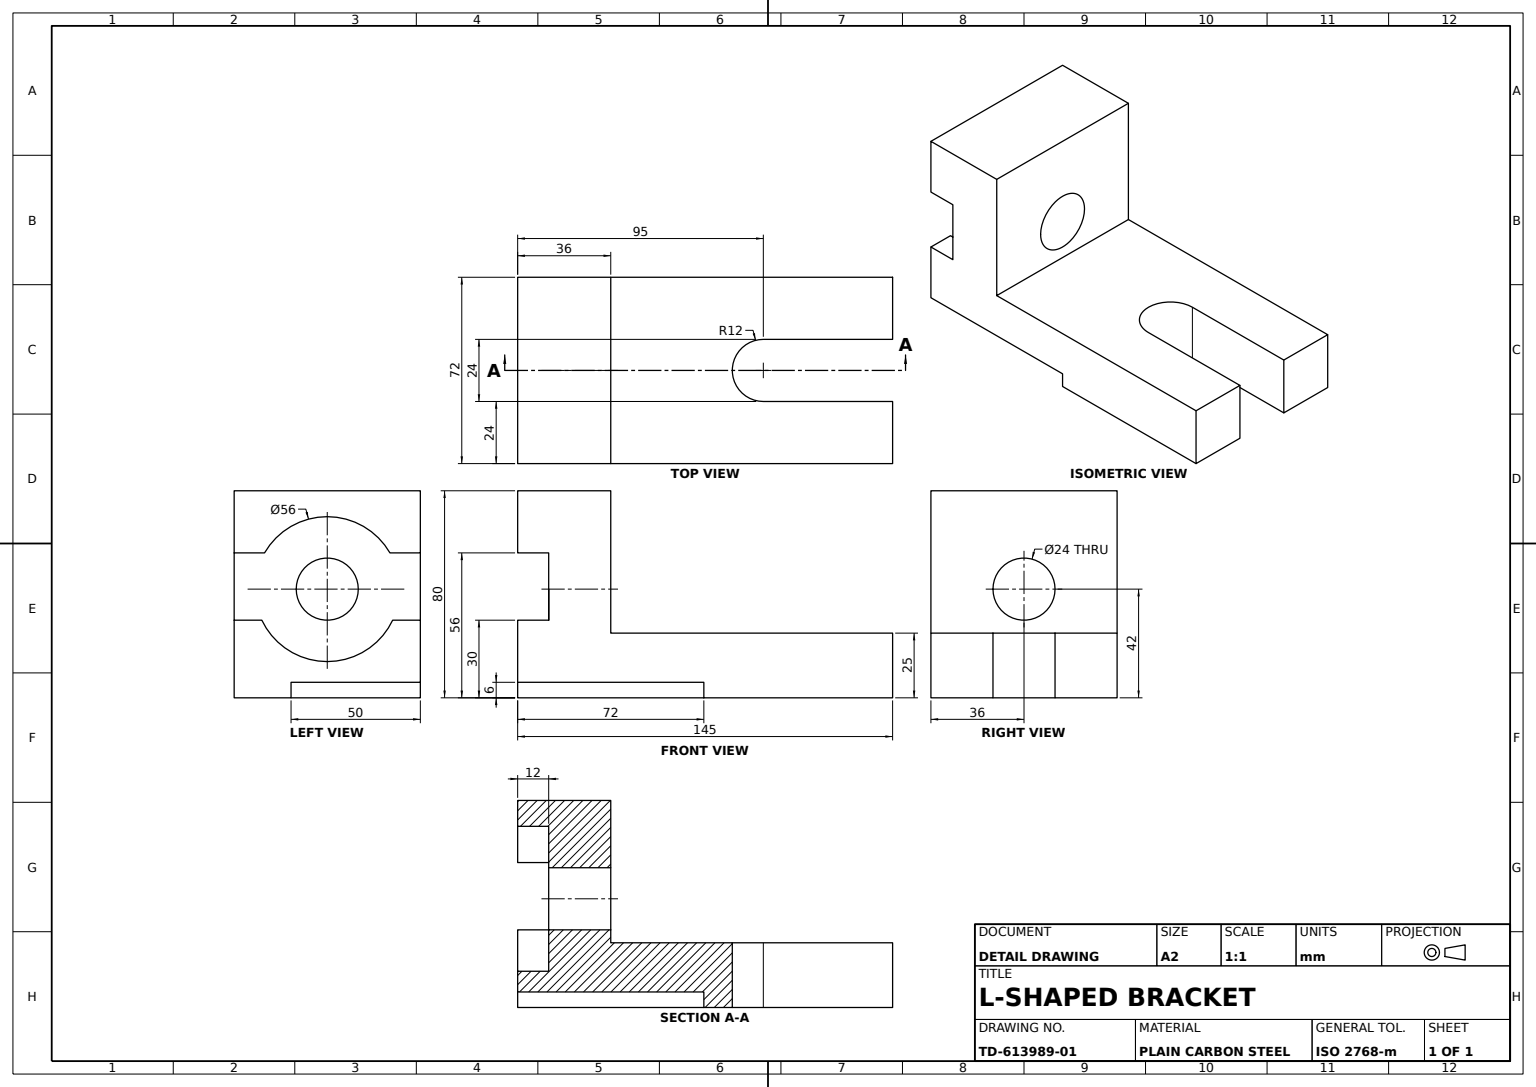
SolidWorks part; units mm, degrees
material "Plain Carbon Steel"
ref_plane "Front Plane" through (0, 0, 0) normal (0, 0, 1) x (1, 0, 0)
ref_plane "Top Plane" through (0, 0, 0) normal (0, 1, 0) x (1, 0, 0)
ref_plane "Right Plane" through (0, 0, 0) normal (1, 0, 0) x (0, 0, -1)
sketch "Base Plate Sketch 145x72" plane through (0, 0, 0) normal (0, 1, 0) x (1, 0, 0)
  line L1 (-72.5, -36) -> (72.5, -36)
  line L2 (-72.5, -36) -> (-72.5, 36)
  line L3 (-72.5, 36) -> (72.5, 36)
  line L4 (72.5, -36) -> (72.5, 36)
  line L5 (-72.5, -36) -> (72.5, 36) construction
  line L6 (-72.5, 36) -> (72.5, -36) construction
  point P0 (0, 0)
  dimension "D1" = 145
  dimension "D2" = 72
extrude "Base Plate 25 Thick" add sketch "Base Plate Sketch 145x72" along normal blind 25
sketch "Underside Relief Sketch" plane through (0, 0, 36) normal (0, 0, 1) x (1, 0, 0)
  line L1 (-72.5, 0) -> (-0.5, 0)
  line L2 (-72.5, 0) -> (-72.5, 6)
  line L3 (-72.5, 6) -> (-0.5, 6)
  line L4 (-0.5, 0) -> (-0.5, 6)
  dimension "D1" = 6
  dimension "D2" = 72
extrude "Underside Relief Cut" cut sketch "Underside Relief Sketch" against normal blind 50
sketch "Clevis Slot Sketch 24 Wide" plane through (0, 25, 0) normal (0, 1, 0) x (1, 0, 0)
  line L0 (72.5, -36) -> (72.5, 36) construction
  line L1 (22.5, 12) -> (72.5, 12)
  line L2 (72.5, 12) -> (72.5, -12)
  line L3 (72.5, -12) -> (22.5, -12)
  arc A0 (22.5, 12) -> (22.5, -12) centre (22.5, 0) ccw
  dimension "D1" = 24
  dimension "D2" = 50
  dimension "D3" = 36
extrude "Clevis Slot Cut" cut sketch "Clevis Slot Sketch 24 Wide" against normal blind 50
sketch "Locating Pad Sketch" plane through (0, 25, 0) normal (0, 1, 0) x (1, 0, 0)
  line L0 (-72.5, -36) -> (72.5, -36) construction
  line L1 (-72.5, 36) -> (-60.5, 36)
  line L2 (-72.5, 36) -> (-72.5, -36)
  line L3 (-72.5, -36) -> (-60.5, -36)
  line L4 (-60.5, 36) -> (-60.5, -36)
  dimension "D1" = 12
extrude "Locating Pad 5 High" add sketch "Locating Pad Sketch" along normal blind 5
sketch "Upright Block Profile Sketch" plane through (0, 0, 36) normal (0, 0, 1) x (1, 0, 0)
  line L0 (-60.5, 25) -> (-60.5, 56)
  line L1 (-60.5, 56) -> (-72.5, 56)
  line L2 (-72.5, 56) -> (-72.5, 80)
  line L3 (-72.5, 80) -> (-36.5, 80)
  line L4 (-36.5, 80) -> (-36.5, 25)
  line L5 (-60.5, 25) -> (72.5, 25) construction
  line L6 (-36.5, 25) -> (-60.5, 25)
  dimension "D1" = 31
  dimension "D2" = 12
  dimension "D3" = 24
  dimension "D4" = 36
extrude "Upright Block 72 Wide" add sketch "Upright Block Profile Sketch" against normal blind 72
sketch "Counterbore Sketch Ø36" plane through (-72.5, 0, 0) normal (-1, 0, 0) x (0, 0, 1)
  circle A0 centre (0, 42) radius 28
  dimension "D1" = 56
  dimension "D2" = 42
  dimension "D3" = 36
extrude "Counterbore Ø36x12" cut sketch "Counterbore Sketch Ø36" against normal blind 12
sketch "Cross Hole Sketch Ø24" plane through (-60.5, 0, 0) normal (-1, 0, 0) x (0, 0, 1)
  circle A0 centre (0, 42) radius 12
  dimension "D1" = 24
extrude "Cross Hole Ø24" cut sketch "Cross Hole Sketch Ø24" against normal through all
